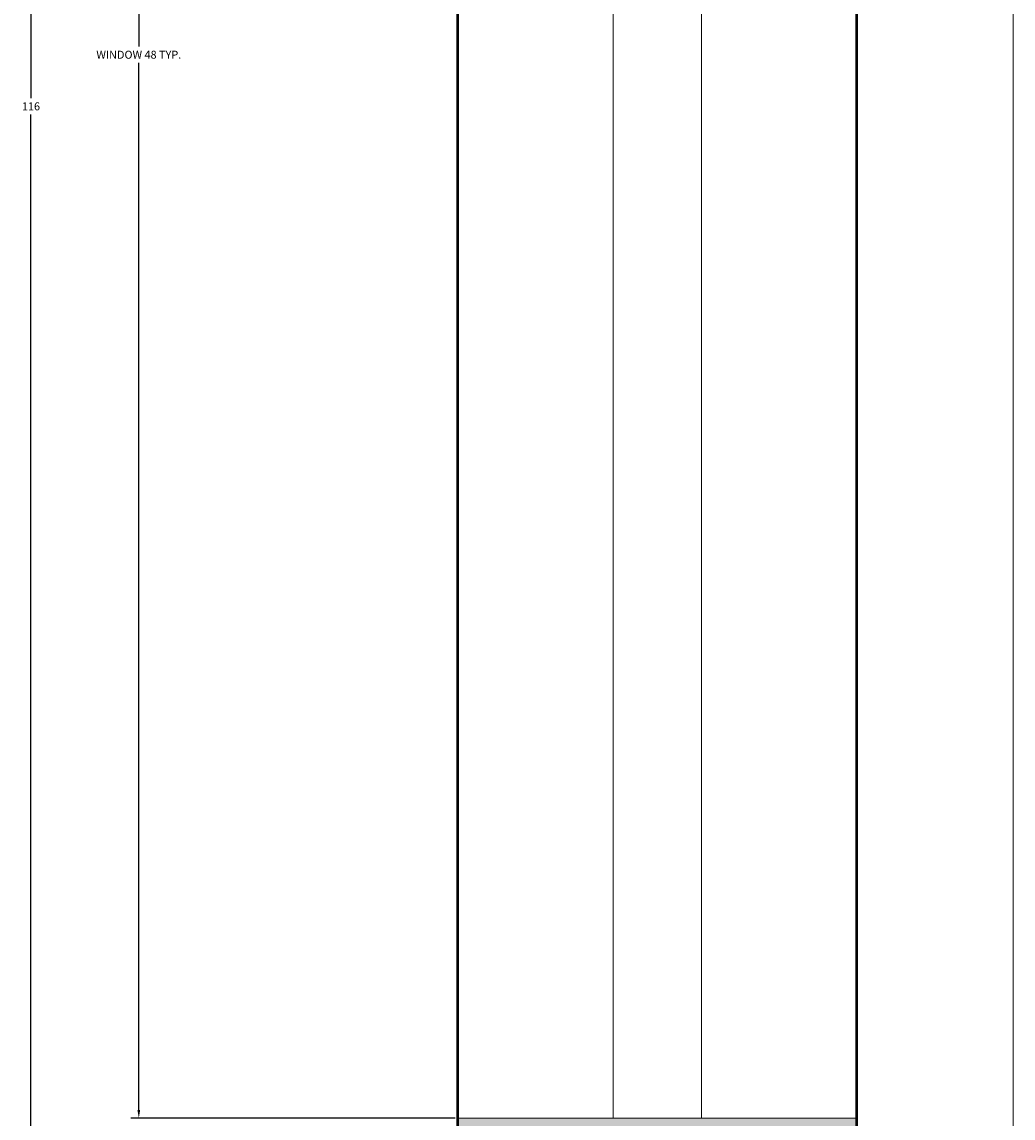
# Model space of a CAD drawing. Units: inches. Extents: x 2231 to 2461, y 2045 to 2455.
# Tile 40 of 95: x 2240 to 2262, y 2222 to 2247. Entities that reach past the tile are written whole.
import ezdxf

# ---------------------------------------------------------------- set-up
doc = ezdxf.new("R2010")
doc.units = ezdxf.units.IN
for name, color, linetype, lineweight in [('A-ANNO-DIMS', 2, 'Continuous', 18), ('A-FURN', 9, 'Continuous', 18), ('A-GLAZ', 4, 'Continuous', 18), ('A-WALL', 7, 'Continuous', 50)]:
    doc.layers.add(name, color=color, linetype=linetype, lineweight=lineweight)
doc.layers.add('A-WALL-PATT', color=18, linetype='Continuous', lineweight=13, true_color=0x000000)
doc.styles.get("Standard").update_dxf_attribs({"font": 'arial.ttf'})
doc.dimstyles.get("Standard").update_dxf_attribs({"dimtxt": 0.18, "dimasz": 0.18, "dimexe": 0.18, "dimexo": 0.0625, "dimgap": 0.09, "dimtad": 0, "dimtih": 1, "dimtoh": 1, "dimdec": 4, "dimzin": 0, "dimdsep": 46, "dimtxsty": 'Standard', "dimcen": 0.09, "dimadec": 0, "dimazin": 0, "dimtfac": 1, "dimtdec": 4, "dimtofl": 0, "dimtmove": 0, "dimatfit": 3, "dimfxl": 1, "dimtolj": 1, "dimtzin": 0, "dimarcsym": 0})

# ---------------------------------------------------------------- blocks, each defined once
blk = doc.blocks.new('WIN-48IN')
for p, q in [((0, 0), (0, 9)), ((48, 9), (48, 0)), ((0, 5.5), (48, 5.5)), ((0, 3.5), (48, 3.5))]:
    blk.add_line(p, q)
blk = doc.blocks.new('*D15')
at = {"layer": 'A-ANNO-DIMS', "color": 0, "lineweight": -2, "transparency": 16777216}
for p, q in [((2249.731, 2269.999), (2242.414, 2269.999)), ((2242.594, 2269.819), (2242.594, 2246.182)), ((2242.594, 2222.179), (2242.594, 2245.816)), ((2249.731, 2221.999), (2242.414, 2221.999))]:
    blk.add_line(p, q, dxfattribs=at)
at = {"layer": 'A-ANNO-DIMS', "color": 0, "transparency": 16777216}
for points in [[(2242.564, 2269.819), (2242.624, 2269.819), (2242.594, 2269.999)], [(2242.564, 2222.179), (2242.624, 2222.179), (2242.594, 2221.999)]]:
    blk.add_solid(points, dxfattribs=at)
at = {"layer": 'Defpoints', "color": 0, "transparency": 16777216}
for p in [(2249.794, 2269.999), (2242.594, 2221.999), (2249.794, 2221.999)]:
    blk.add_point(p, dxfattribs=at)
at = {"layer": 'A-ANNO-DIMS', "color": 0, "transparency": 16777216, "insert": (2242.594, 2245.999), "char_height": 0.18, "attachment_point": 5}
blk.add_mtext('\\A1;WINDOW 48 TYP.', dxfattribs=at)
blk = doc.blocks.new('*D16')
at = {"layer": 'A-ANNO-DIMS', "color": 0, "lineweight": -2, "transparency": 16777216}
for p, q in [((2249.794, 2221.937), (2249.794, 2214.619)), ((2258.794, 2221.937), (2258.794, 2214.619)), ((2249.974, 2214.799), (2253.835, 2214.799)), ((2258.614, 2214.799), (2254.752, 2214.799))]:
    blk.add_line(p, q, dxfattribs=at)
at = {"layer": 'A-ANNO-DIMS', "color": 0, "transparency": 16777216}
for points in [[(2249.974, 2214.829), (2249.974, 2214.769), (2249.794, 2214.799)], [(2258.614, 2214.829), (2258.614, 2214.769), (2258.794, 2214.799)]]:
    blk.add_solid(points, dxfattribs=at)
at = {"layer": 'Defpoints', "color": 0, "transparency": 16777216}
for p in [(2249.794, 2221.999), (2258.794, 2221.999), (2258.794, 2214.799)]:
    blk.add_point(p, dxfattribs=at)
at = {"layer": 'A-ANNO-DIMS', "color": 0, "transparency": 16777216, "insert": (2254.294, 2214.799), "char_height": 0.18, "attachment_point": 5}
blk.add_mtext('\\A1;9 TYP.', dxfattribs=at)
blk = doc.blocks.new('*D40')
at = {"layer": 'A-ANNO-DIMS', "color": 0, "lineweight": -2, "transparency": 16777216}
for p, q in [((2258.731, 2302.833), (2239.981, 2302.833)), ((2240.161, 2302.653), (2240.161, 2245.015)), ((2240.161, 2187.013), (2240.161, 2244.651)), ((2258.731, 2186.833), (2239.981, 2186.833))]:
    blk.add_line(p, q, dxfattribs=at)
at = {"layer": 'A-ANNO-DIMS', "color": 0, "transparency": 16777216}
for points in [[(2240.131, 2302.653), (2240.191, 2302.653), (2240.161, 2302.833)], [(2240.131, 2187.013), (2240.191, 2187.013), (2240.161, 2186.833)]]:
    blk.add_solid(points, dxfattribs=at)
at = {"layer": 'Defpoints', "color": 0, "transparency": 16777216}
for p in [(2240.161, 2302.833), (2258.794, 2302.833), (2258.794, 2186.833)]:
    blk.add_point(p, dxfattribs=at)
at = {"layer": 'A-ANNO-DIMS', "color": 0, "transparency": 16777216, "insert": (2240.161, 2244.833), "char_height": 0.18, "attachment_point": 5}
blk.add_mtext('\\A1;116', dxfattribs=at)
blk = doc.blocks.new('*D47')
at = {"layer": 'A-ANNO-DIMS', "color": 0, "lineweight": -2, "transparency": 16777216}
for p, q in [((2258.794, 2182.895), (2258.794, 2454.645)), ((2258.974, 2454.465), (2276.575, 2454.465)), ((2294.614, 2454.465), (2277.012, 2454.465)), ((2294.794, 2182.895), (2294.794, 2454.645))]:
    blk.add_line(p, q, dxfattribs=at)
at = {"layer": 'A-ANNO-DIMS', "color": 0, "transparency": 16777216}
for points in [[(2258.974, 2454.495), (2258.974, 2454.435), (2258.794, 2454.465)], [(2294.614, 2454.495), (2294.614, 2454.435), (2294.794, 2454.465)]]:
    blk.add_solid(points, dxfattribs=at)
at = {"layer": 'Defpoints', "color": 0, "transparency": 16777216}
for p in [(2294.794, 2454.465), (2258.794, 2182.833), (2294.794, 2182.833)]:
    blk.add_point(p, dxfattribs=at)
at = {"layer": 'A-ANNO-DIMS', "color": 0, "transparency": 16777216, "insert": (2276.794, 2454.465), "char_height": 0.18, "attachment_point": 5}
blk.add_mtext('\\A1;36', dxfattribs=at)
blk = doc.blocks.new('*D51')
at = {"layer": 'A-ANNO-DIMS', "color": 0, "lineweight": -2, "transparency": 16777216}
for p, q in [((2258.794, 2306.77), (2258.794, 2044.803)), ((2330.794, 2306.77), (2330.794, 2044.803)), ((2258.974, 2044.983), (2294.576, 2044.983)), ((2330.614, 2044.983), (2295.011, 2044.983))]:
    blk.add_line(p, q, dxfattribs=at)
at = {"layer": 'A-ANNO-DIMS', "color": 0, "transparency": 16777216}
for points in [[(2258.974, 2045.013), (2258.974, 2044.953), (2258.794, 2044.983)], [(2330.614, 2045.013), (2330.614, 2044.953), (2330.794, 2044.983)]]:
    blk.add_solid(points, dxfattribs=at)
at = {"layer": 'Defpoints', "color": 0, "transparency": 16777216}
for p in [(2258.794, 2306.833), (2330.794, 2306.833), (2330.794, 2044.983)]:
    blk.add_point(p, dxfattribs=at)
at = {"layer": 'A-ANNO-DIMS', "color": 0, "transparency": 16777216, "insert": (2294.794, 2044.983), "char_height": 0.18, "attachment_point": 5}
blk.add_mtext('\\A1;72', dxfattribs=at)

msp = doc.modelspace()

# ---------------------------------------------------------------- hatches: boundary and pattern name
at = {"layer": 'A-WALL-PATT'}
h = msp.add_hatch(color=256, dxfattribs=at)
h.dxf.hatch_style = 1
h.paths.add_polyline_path([(2441.7935, 2269.1535), (2432.7935, 2269.1535), (2432.7935, 2186.8328), (2396.7935, 2186.8328), (2396.7935, 2286.8328), (2394.7935, 2286.8328), (2394.7935, 2186.8328), (2334.7935, 2186.8328), (2334.7935, 2182.8328), (2432.7935, 2182.8328), (2432.7935, 2072.8328), (2416.6639, 2072.8328), (2416.6639, 2063.8328), (2441.7935, 2063.8328)])
h.paths.add_polyline_path([(2368.6639, 2072.8328), (2367.04, 2072.8328), (2330.7942, 2072.8328), (2330.7397, 2063.8328), (2368.6639, 2063.8328)])
h.paths.add_polyline_path([(2300.7392, 2068.3328), (2300.7392, 2072.8328), (2298.7935, 2072.8328), (2294.7935, 2072.8328), (2258.7935, 2072.8328), (2258.7935, 2120.8328), (2294.7935, 2120.8328), (2298.7935, 2120.8328), (2298.7935, 2128.8328), (2294.7935, 2128.8328), (2294.7935, 2124.8328), (2258.7935, 2124.8328), (2258.7935, 2182.8328), (2294.7935, 2182.8328), (2294.7935, 2174.8328), (2298.7935, 2174.8328), (2298.7935, 2182.8328), (2304.7935, 2182.8328), (2304.7935, 2186.8328), (2258.7935, 2186.8328), (2258.7935, 2221.999), (2249.7935, 2221.999), (2249.7935, 2063.8328), (2300.7392, 2063.8328)])
h.paths.add_polyline_path([(2391.9338, 2435.8328), (2333.82, 2435.8328), (2333.82, 2426.8328), (2368.7935, 2426.8328), (2368.7935, 2374.9508), (2368.7935, 2370.8328), (2372.3935, 2370.8328), (2372.7935, 2370.8328), (2372.7935, 2426.8328), (2391.9338, 2426.8328)])
h.paths.add_polyline_path([(2441.7935, 2435.8328), (2415.9338, 2435.8328), (2415.9338, 2426.8328), (2432.7935, 2426.8328), (2432.7935, 2334.8328), (2372.7935, 2334.8328), (2372.7935, 2346.8328), (2368.7935, 2346.8328), (2368.7935, 2306.8328), (2360.7935, 2306.8328), (2360.7935, 2302.8328), (2368.7935, 2302.8328), (2372.7935, 2302.8328), (2372.7935, 2330.8328), (2432.7935, 2330.8328), (2432.7935, 2317.1535), (2441.7935, 2317.1535)])
h.paths.add_polyline_path([(2285.82, 2435.8328), (2249.7935, 2435.8328), (2249.7935, 2269.999), (2258.7935, 2269.999), (2258.7935, 2302.8328), (2318.8168, 2302.8328), (2330.7935, 2302.8328), (2330.7935, 2306.8328), (2258.7935, 2306.8328), (2258.7935, 2426.8328), (2285.82, 2426.8328)])

# ---------------------------------------------------------------- linework, layer by layer
at = {"layer": 'A-FURN'}
msp.add_line((2262.3207, 2255.1137), (2262.3207, 2195.1137), dxfattribs=at)
at = {"layer": 'A-WALL'}
msp.add_line((2258.7935, 2186.8328), (2258.7935, 2302.8328), dxfattribs=at)
msp.add_lwpolyline([(2300.7392, 2063.8328), (2249.7935, 2063.8328), (2249.7935, 2435.8328), (2441.7935, 2435.8328), (2441.7935, 2063.8328), (2330.7397, 2063.8328)], dxfattribs=at)

# ---------------------------------------------------------------- block references
at = {"layer": 'A-GLAZ', "rotation": 270.000000000001}
msp.add_blockref('WIN-48IN', (2249.7937, 2269.999), dxfattribs=at)

# ---------------------------------------------------------------- dimensions: what is measured, and where the dimension line sits
at = {"layer": 'A-ANNO-DIMS'}
for base, p1, p2, picture, middle in [((2294.7935, 2454.4653), (2258.7935, 2182.8328), (2294.7935, 2182.8328), '*D47', (2276.7935, 2454.4653)), ((2330.7935, 2044.9825), (2258.7935, 2306.8328), (2330.7935, 2306.8328), '*D51', (2294.7935, 2044.9825))]:
    dim = msp.add_linear_dim(base=base, p1=p1, p2=p2, dimstyle='Standard', override={"dimdec": 0, "dimlfac": 1, "dimrnd": 0, "dimzin": 0, "dimdsep": 46, "dimlunit": 2}, dxfattribs=at)
    dim.commit()
    dim.dimension.update_dxf_attribs({"geometry": picture, "text_midpoint": middle})
dim = msp.add_linear_dim(base=(2240.161, 2302.8328), p1=(2258.7935, 2186.8328), p2=(2258.7935, 2302.8328), angle=90, dimstyle='Standard', override={"dimdec": 0, "dimlfac": 1, "dimrnd": 0, "dimzin": 0, "dimdsep": 46, "dimlunit": 2}, dxfattribs=at)
dim.commit()
dim.dimension.update_dxf_attribs({"geometry": '*D40', "text_midpoint": (2240.161, 2244.8328)})
dim = msp.add_linear_dim(base=(2242.5935, 2221.999), p1=(2249.7935, 2269.999), p2=(2249.7935, 2221.999), angle=270, text='WINDOW <> TYP.', dimstyle='Standard', override={"dimdec": 0, "dimlfac": 1, "dimrnd": 0, "dimzin": 0, "dimdsep": 46, "dimlunit": 2}, dxfattribs=at)
dim.commit()
dim.dimension.update_dxf_attribs({"geometry": '*D15', "text_midpoint": (2242.5935, 2245.999)})
dim = msp.add_linear_dim(base=(2258.7935, 2214.799), p1=(2249.7935, 2221.999), p2=(2258.7935, 2221.999), text='<> TYP.', dimstyle='Standard', override={"dimdec": 0, "dimlfac": 1, "dimrnd": 0, "dimzin": 0, "dimdsep": 46, "dimlunit": 2}, dxfattribs=at)
dim.commit()
dim.dimension.update_dxf_attribs({"geometry": '*D16', "text_midpoint": (2254.2935, 2214.799)})

doc.saveas('drawing.dxf')
